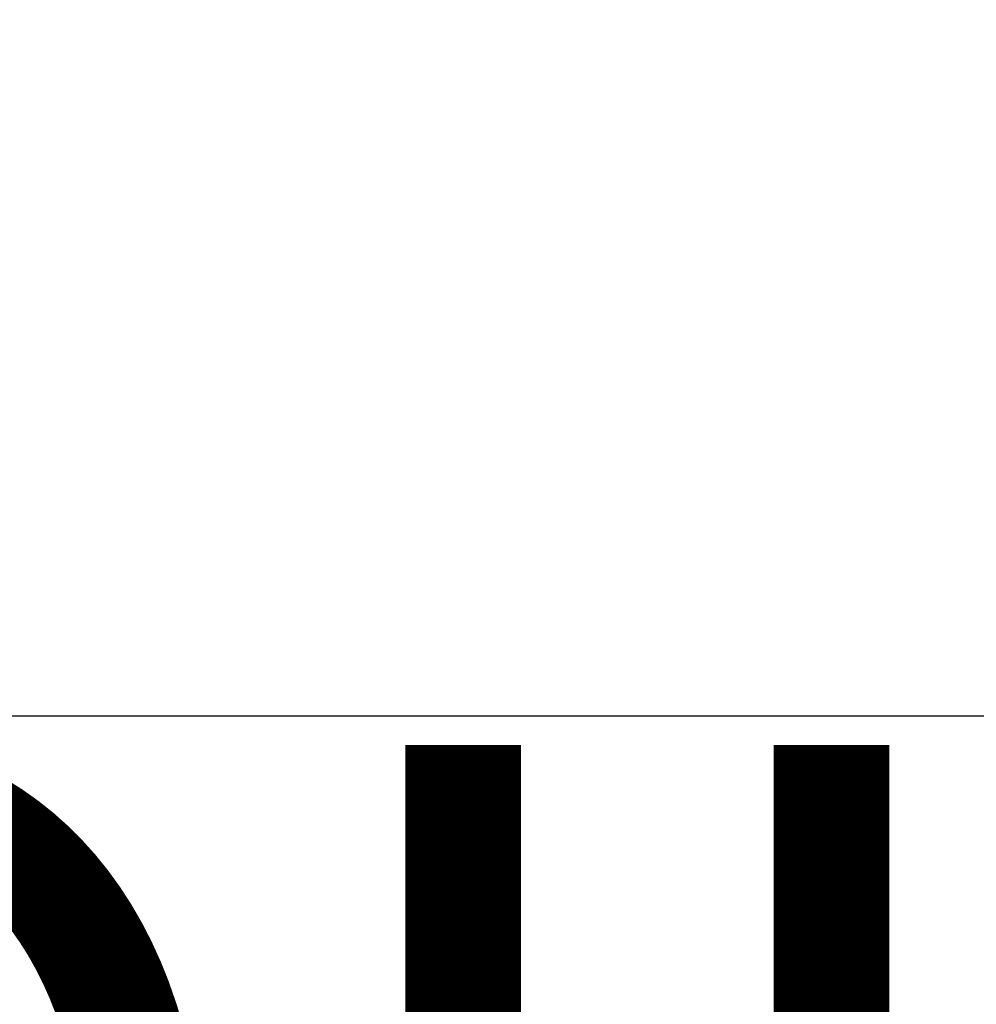
# Model space of a CAD drawing. Units: inches. Extents: x 2696 to 3240, y 1564 to 2310.
# Tile 18 of 76: x 2783.067 to 2792.41, y 1890.388 to 1900.004. Entities that reach past the tile are written whole.
import ezdxf

# ---------------------------------------------------------------- set-up
doc = ezdxf.new("R2010")
doc.units = ezdxf.units.IN
doc.layers.add('A-ANNO-DIMS', color=3, linetype='Continuous', lineweight=18)
doc.layers.add('A-AREA-IDEN', color=7, linetype='Continuous', lineweight=18)
doc.styles.add('TIMES NEW', font='times.ttf')
doc.styles.add('YQ_DIM', font='SUPEROS.SHX', dxfattribs={"width": 0.8, "bigfont": 'HZDX.SHX'})
doc.dimstyles.new('Siddhuu', dxfattribs={"dimtxt": 6, "dimasz": 2.5, "dimexe": 1.25, "dimexo": 0.625, "dimtad": 1, "dimdec": 1, "dimlunit": 4, "dimtxsty": 'TIMES NEW', "dimcen": 2.5, "dimclrd": 256, "dimclre": 1, "dimclrt": 7, "dimadec": 0, "dimazin": 0, "dimtfac": 1, "dimtdec": 1, "dimtmove": 0, "dimatfit": 3, "dimfxl": 1, "dimtolj": 1, "dimlwd": -1, "dimarcsym": 0})

# ---------------------------------------------------------------- blocks, each defined once
blk = doc.blocks.new('*D55')
at = {"layer": 'A-ANNO-DIMS', "color": 1, "lineweight": -2, "transparency": 16777216}
for p, q in [((3189.9864, 1980.2011), (2709.3614, 1980.2011)), ((3189.9864, 1893.2011), (2709.3614, 1893.2011))]:
    blk.add_line(p, q, dxfattribs=at)
at = {"layer": 'A-ANNO-DIMS', "transparency": 16777216}
blk.add_line((2710.6114, 1895.7011), (2710.6114, 1977.7011), dxfattribs=at)
for points in [[(2710.1947, 1977.7011), (2711.0281, 1977.7011), (2710.6114, 1980.2011)], [(2710.1947, 1895.7011), (2711.0281, 1895.7011), (2710.6114, 1893.2011)]]:
    blk.add_solid(points, dxfattribs=at)
at = {"layer": 'Defpoints', "color": 0, "transparency": 16777216}
for p in [(2710.6114, 1980.2011), (3190.6114, 1980.2011), (3190.6114, 1893.2011)]:
    blk.add_point(p, dxfattribs=at)
at = {"layer": 'A-ANNO-DIMS', "color": 7, "transparency": 16777216, "insert": (2706.9258, 1936.7011), "char_height": 6, "attachment_point": 5, "rotation": 90, "style": 'TIMES NEW'}
blk.add_mtext('\\A1;7\'-3"', dxfattribs=at)
blk = doc.blocks.new('*D57')
at = {"layer": 'A-ANNO-DIMS', "color": 1, "lineweight": -2, "transparency": 16777216}
for p, q in [((2754.6114, 2018.5761), (2754.6114, 1568.9511)), ((2956.7088, 2018.5761), (2956.7088, 1568.9511))]:
    blk.add_line(p, q, dxfattribs=at)
at = {"layer": 'A-ANNO-DIMS', "transparency": 16777216}
blk.add_line((2757.1114, 1570.2011), (2954.2088, 1570.2011), dxfattribs=at)
for points in [[(2757.1114, 1570.6178), (2757.1114, 1569.7844), (2754.6114, 1570.2011)], [(2954.2088, 1570.6178), (2954.2088, 1569.7844), (2956.7088, 1570.2011)]]:
    blk.add_solid(points, dxfattribs=at)
at = {"layer": 'Defpoints', "color": 0, "transparency": 16777216}
for p in [(2754.6114, 2019.2011), (2956.7088, 2019.2011), (2956.7088, 1570.2011)]:
    blk.add_point(p, dxfattribs=at)
at = {"layer": 'A-ANNO-DIMS', "color": 7, "transparency": 16777216, "insert": (2855.6601, 1573.878), "char_height": 6, "attachment_point": 5, "style": 'TIMES NEW'}
blk.add_mtext('\\A1;16\'-10"', dxfattribs=at)
blk = doc.blocks.new('*D78')
at = {"layer": 'A-ANNO-DIMS', "transparency": 16777216}
for p, q in [((2710.6114, 1901.7011), (2710.6114, 1935.1007)), ((2710.6114, 1895.7011), (2710.6114, 1899.2011))]:
    blk.add_line(p, q, dxfattribs=at)
at = {"layer": 'A-ANNO-DIMS', "color": 1, "lineweight": -2, "transparency": 16777216}
for p, q in [((3189.9864, 1901.7011), (2709.3614, 1901.7011)), ((3189.9864, 1893.2011), (2709.3614, 1893.2011))]:
    blk.add_line(p, q, dxfattribs=at)
at = {"layer": 'A-ANNO-DIMS', "transparency": 16777216}
for points in [[(2710.1947, 1899.2011), (2711.0281, 1899.2011), (2710.6114, 1901.7011)], [(2710.1947, 1895.7011), (2711.0281, 1895.7011), (2710.6114, 1893.2011)]]:
    blk.add_solid(points, dxfattribs=at)
at = {"layer": 'Defpoints', "color": 0, "transparency": 16777216}
for p in [(2710.6114, 1901.7011), (3190.6114, 1901.7011), (3190.6114, 1893.2011)]:
    blk.add_point(p, dxfattribs=at)
at = {"layer": 'A-ANNO-DIMS', "color": 7, "transparency": 16777216, "insert": (2706.8501, 1919.6509), "char_height": 6, "attachment_point": 5, "rotation": 90, "style": 'TIMES NEW'}
blk.add_mtext('\\A1;0\'-8 1/2"', dxfattribs=at)

msp = doc.modelspace()

# ---------------------------------------------------------------- texts
at = {"layer": 'A-AREA-IDEN', "insert": (2769.1285, 1892.921), "char_height": 9, "attachment_point": 1, "style": 'YQ_DIM'}
msp.add_mtext_dynamic_manual_height_columns('TOILET\\P5\'X5\'4.5"', width=48.003243, gutter_width=12.5, heights=[0], dxfattribs=at)

# ---------------------------------------------------------------- dimensions: what is measured, and where the dimension line sits
at = {"layer": 'A-ANNO-DIMS'}
dim = msp.add_linear_dim(base=(2956.7088, 1570.2011), p1=(2754.6114, 2019.2011), p2=(2956.7088, 2019.2011), dimstyle='Siddhuu', override={"dimdec": 1, "dimlfac": 1, "dimrnd": 0, "dimzin": 1, "dimdsep": 46, "dimlunit": 4, "dimfrac": 2}, dxfattribs=at)
dim.commit()
dim.dimension.update_dxf_attribs({"geometry": '*D57', "text_midpoint": (2855.6601, 1573.878)})
for base, p2, picture, middle in [((2710.6114, 1980.2011), (3190.6114, 1980.2011), '*D55', (2706.9258, 1936.7011)), ((2710.6114, 1901.7011), (3190.6114, 1901.7011), '*D78', (2706.8501, 1919.6509))]:
    dim = msp.add_linear_dim(base=base, p1=(3190.6114, 1893.2011), p2=p2, angle=90, dimstyle='Siddhuu', override={"dimdec": 1, "dimlfac": 1, "dimrnd": 0, "dimzin": 1, "dimdsep": 46, "dimlunit": 4, "dimfrac": 2}, dxfattribs=at)
    dim.commit()
    dim.dimension.update_dxf_attribs({"geometry": picture, "text_midpoint": middle})

doc.saveas('drawing.dxf')
